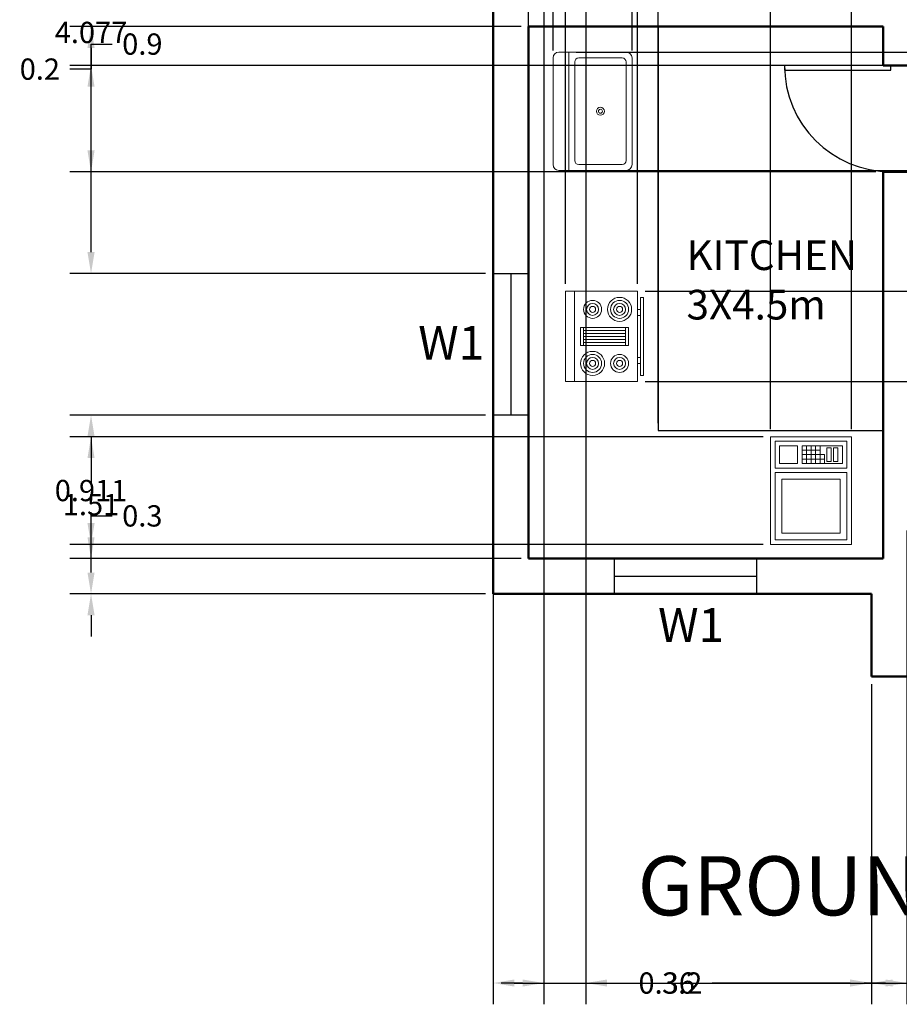
# Model space of a CAD drawing. Units: metres. Extents: x 2443.7 to 2482.9, y 2261.4 to 2287.
# Tile 1 of 8: x 2443.7 to 2451.1, y 2261.4 to 2269.7. Entities that reach past the tile are written whole.
import ezdxf

# ---------------------------------------------------------------- set-up
doc = ezdxf.new("R2010")
doc.units = ezdxf.units.M
for name, color, linetype, lineweight in [('A-ANNO-DIMS', 2, 'Continuous', 18), ('A-AREA-IDEN', 11, 'Continuous', 25), ('A-EQPM', 20, 'Continuous', 18), ('A-FLOR-CASE', 20, 'Continuous', 25), ('A-FLOR-FIXT', 20, 'Continuous', 18), ('A-MODL', 7, 'Continuous', 25), ('A-WALL', 7, 'Continuous', 50), ('door', 6, 'Continuous', 25), ('text', 11, 'Continuous', 25), ('window', 3, 'Continuous', 25)]:
    doc.layers.add(name, color=color, linetype=linetype, lineweight=lineweight)
doc.styles.get("Standard").update_dxf_attribs({"font": 'arial.ttf'})
doc.dimstyles.get("Standard").update_dxf_attribs({"dimtxt": 0.18, "dimasz": 0.18, "dimexe": 0.18, "dimexo": 0.0625, "dimgap": 0.09, "dimtad": 0, "dimtih": 1, "dimtoh": 1, "dimdec": 4, "dimzin": 0, "dimdsep": 46, "dimtxsty": 'Standard', "dimcen": 0.09, "dimadec": 0, "dimazin": 0, "dimtfac": 1, "dimtdec": 4, "dimtofl": 0, "dimtmove": 0, "dimatfit": 3, "dimfxl": 1, "dimtolj": 1, "dimtzin": 0, "dimarcsym": 0})

# ---------------------------------------------------------------- blocks, each defined once
blk = doc.blocks.new('*U2')
for p, q in [((0, 0), (0, -6)), ((-40, 0), (-40, -6))]:
    blk.add_line(p, q)
blk.add_lwpolyline([(0, 0), (0, 40), (-1.75, 40), (-1.75, 0)], close=True)
blk.add_arc((0, 0), 40, 90, 180)
blk = doc.blocks.new('Microwave')
for p, q in [((19, 7), (19, 11)), ((20, 11), (20, 7)), ((21, 7), (21, 11)), ((18, 10), (22, 10)), ((22, 9), (18, 9)), ((18, 8), (22, 8)), ((22, 7), (18, 7)), ((19, 6), (19, 7)), ((20, 7), (20, 6)), ((20, 6), (18, 6))]:
    blk.add_line(p, q)
for points in [[(0, 0), (0, 18), (24, 18), (24, 0)], [(1, 1), (1, 17), (16, 17), (16, 1)], [(2.5, 2.5), (2.5, 15.5), (14.5, 15.5), (14.5, 2.5)], [(17, 1), (17, 17), (23, 17), (23, 1)], [(18, 12), (18, 16), (22, 16), (22, 12)], [(18, 2), (18, 11), (22, 11), (22, 2)], [(18.5, 4.5), (18.5, 5.5), (21.5, 5.5), (21.5, 4.5)], [(18.5, 3), (18.5, 4), (21.5, 4), (21.5, 3)]]:
    blk.add_lwpolyline(points, close=True)
blk = doc.blocks.new('Range-Oven - 30 in top')
for p, q in [((0, -3), (30, -3)), ((12, -6), (18, -6)), ((13, -20), (13, -6)), ((14, -6), (14, -20)), ((15, -20), (15, -6)), ((16, -6), (16, -20)), ((17, -20), (17, -6)), ((18, -20), (12, -20)), ((6, -24), (6, -25)), ((8, -25), (8, -24)), ((22, -25), (22, -24)), ((24, -24), (24, -25))]:
    blk.add_line(p, q)
for points in [[(0, -24), (0, 0), (30, 0), (30, -24)], [(12, -21), (12, -5), (18, -5), (18, -21)], [(2, -26), (2, -25), (28, -25), (28, -26)]]:
    blk.add_lwpolyline(points, close=True)
for centre, radius in [((6, -9), 4), ((6, -9), 3), ((24, -9), 3), ((6, -9), 2), ((6, -9), 1), ((24, -9), 2), ((24, -9), 1), ((6, -18), 3), ((6, -18), 2), ((24, -18), 4), ((24, -18), 3), ((24, -18), 2), ((6, -18), 1), ((24, -18), 1)]:
    blk.add_circle(centre, radius)
blk = doc.blocks.new('Sink-single - 30 in top')
blk.add_line((-15, -3.999996), (15, -3.999996))
for points in [[(-13.5, 0), (13.5, 0)], [(-15, -18.499996), (-15, -1.5)], [(15, -1.5), (15, -18.499996)], [(-13.5, -17.499996), (-13.5, -6.499996)], [(-12.5, -5.499996), (12.5, -5.499996)], [(13.5, -6.499996), (13.5, -17.499996)], [(12.5, -18.499996), (-12.5, -18.499996)], [(13.5, -19.999996), (-13.5, -19.999996)]]:
    blk.add_lwpolyline(points)
for radius in [1, 0.5]:
    blk.add_circle((0, -11.999996), radius)
for centre, radius, start, end in [((-13.5, -1.5), 1.5, 90, 180), ((13.5, -1.5), 1.5, 0, 90), ((-12.5, -6.499996), 1, 90, 180), ((12.5, -6.499996), 1, 0, 90), ((-13.5, -18.499996), 1.5, 180, 270), ((-12.5, -17.499996), 1, 180, 270), ((12.5, -17.499996), 1, 270, 0), ((13.5, -18.499996), 1.5, 270, 0)]:
    blk.add_arc(centre, radius, start, end)
blk = doc.blocks.new('aditya')
at = {"layer": 'A-FLOR-CASE'}
for points in [[(1.3977, 0.3), (0.3, 0.3), (0.3, 4.8), (1.3977, 4.8), (1.3977, 1.3826)], [(1.3977, 1.3826), (3.3, 1.3826), (3.3, 0.3), (0.3, 0.3), (0.3, 1.3826)]]:
    blk.add_lwpolyline(points, dxfattribs=at)
at = {"layer": 'A-WALL'}
for p, q in [((0, 0), (0, 9.9)), ((0.3, 0.3), (0.3, 4.8)), ((0.3, 4.8), (3.3, 4.8)), ((3.3, 4.4718), (3.3, 4.8)), ((3.3, 0.3), (3.3, 3.5742)), ((0.3, 0.3), (3.3, 0.3)), ((0, 0), (3.2, 0)), ((3.2, -0.4), (3.2, 0)), ((3.2, -0.7), (3.2, 0)), ((3.5, -0.7), (3.2, -0.7))]:
    blk.add_line(p, q, dxfattribs=at)
for points in [[(3.3, 4.4718), (3.5, 4.4718)], [(3.5, 3.5718), (3.3, 3.5718), (3.3, 3.5742)]]:
    blk.add_lwpolyline(points, dxfattribs=at)
at = {"layer": 'window'}
for p, q in [((0.15, 2.7118), (0.15, 1.5118)), ((1.0287, 0.15), (2.2287, 0.15))]:
    blk.add_line(p, q, dxfattribs=at)
for points in [[(0, 2.7118), (0.3, 2.7118), (0.3, 1.5118), (0, 1.5118)], [(1.0287, 0), (1.0287, 0.3), (2.2287, 0.3), (2.2287, 0)]]:
    blk.add_lwpolyline(points, close=True, dxfattribs=at)
at = {"layer": 'A-EQPM', "rotation": 90}
for name, p, xscale, yscale, zscale in [('Range-Oven - 30 in top', (0.6135, 1.798), 0.0254, 0.0254, 0.0254), ('Microwave', (3.0315, 0.4191), 0.0379607650173663, 0.0379607650173663, 0.0379607650173663)]:
    blk.add_blockref(name, p, dxfattribs=dict(at, xscale=xscale, yscale=yscale, zscale=zscale))
at = {"layer": 'A-FLOR-FIXT', "xscale": 0.0333950198631644, "yscale": 0.0333950198631644, "zscale": 0.0333950198631644, "rotation": 90}
blk.add_blockref('Sink-single - 30 in top', (0.5076, 4.0837), dxfattribs=at)
at = {"layer": 'door', "xscale": 0.0224999999999983, "yscale": 0.0224999999999983, "zscale": 0.0224999999999983, "rotation": 90}
blk.add_blockref('*U2', (3.365, 4.4718), dxfattribs=at)
at = {"layer": 'A-AREA-IDEN', "insert": (1.6365, 2.991), "char_height": 0.250924, "attachment_point": 1}
blk.add_mtext_dynamic_manual_height_columns('{\\fArial|b1|i1|c0|p34;KITCHEN\\P3X4.5m}', width=10.569305, gutter_width=7.8414, heights=[0], dxfattribs=at)
at = {"layer": 'text'}
for p in [(-0.6327, 1.9824), (1.3964, -0.4055)]:
    blk.add_text('W1', height=0.28528, dxfattribs=at).set_placement(p)
at = {"layer": 'text', "insert": (1.2226, -2.2194), "char_height": 0.5, "attachment_point": 1}
blk.add_mtext_dynamic_manual_height_columns('{\\fArial|b1|i1|c0|p34;GROUND FLOOR PLAN}', width=17.015787, gutter_width=7.8414, heights=[0], dxfattribs=at)
blk = doc.blocks.new('*D22')
at = {"layer": 'A-ANNO-DIMS', "color": 0, "lineweight": -2, "transparency": 16777216}
for p, q in [((2457.8828, 2265.0972), (2457.8828, 2261.3876)), ((2447.6828, 2264.7972), (2447.6828, 2261.3876)), ((2447.8628, 2261.5676), (2452.4684, 2261.5676)), ((2457.7028, 2261.5676), (2453.0971, 2261.5676))]:
    blk.add_line(p, q, dxfattribs=at)
at = {"layer": 'A-ANNO-DIMS', "color": 0, "transparency": 16777216}
for points in [[(2447.8628, 2261.5976), (2447.8628, 2261.5376), (2447.6828, 2261.5676)], [(2457.7028, 2261.5976), (2457.7028, 2261.5376), (2457.8828, 2261.5676)]]:
    blk.add_solid(points, dxfattribs=at)
at = {"layer": 'Defpoints', "color": 0, "transparency": 16777216}
for p in [(2457.8828, 2265.1597), (2447.6828, 2264.8597), (2457.8828, 2261.5676)]:
    blk.add_point(p, dxfattribs=at)
at = {"layer": 'A-ANNO-DIMS', "color": 0, "transparency": 16777216, "insert": (2452.7828, 2261.5676), "char_height": 0.18, "attachment_point": 5}
blk.add_mtext('\\A1;10.2', dxfattribs=at)
blk = doc.blocks.new('*D24')
at = {"layer": 'A-ANNO-DIMS', "color": 0, "lineweight": -2, "transparency": 16777216}
for p, q in [((2447.6828, 2264.7972), (2447.6828, 2261.3876)), ((2450.8828, 2264.0972), (2450.8828, 2261.3876)), ((2447.8628, 2261.5676), (2449.0299, 2261.5676)), ((2450.7028, 2261.5676), (2449.5356, 2261.5676))]:
    blk.add_line(p, q, dxfattribs=at)
at = {"layer": 'A-ANNO-DIMS', "color": 0, "transparency": 16777216}
for points in [[(2447.8628, 2261.5976), (2447.8628, 2261.5376), (2447.6828, 2261.5676)], [(2450.7028, 2261.5976), (2450.7028, 2261.5376), (2450.8828, 2261.5676)]]:
    blk.add_solid(points, dxfattribs=at)
at = {"layer": 'Defpoints', "color": 0, "transparency": 16777216}
for p in [(2447.6828, 2264.8597), (2450.8828, 2264.1597), (2450.8828, 2261.5676)]:
    blk.add_point(p, dxfattribs=at)
at = {"layer": 'A-ANNO-DIMS', "color": 0, "transparency": 16777216, "insert": (2449.2828, 2261.5676), "char_height": 0.18, "attachment_point": 5}
blk.add_mtext('\\A1;3.2', dxfattribs=at)
blk = doc.blocks.new('*D25')
at = {"layer": 'A-ANNO-DIMS', "color": 0, "lineweight": -2, "transparency": 16777216}
for p, q in [((2450.8828, 2264.0972), (2450.8828, 2261.3876)), ((2453.5828, 2264.0972), (2453.5828, 2261.3876)), ((2451.0628, 2261.5676), (2451.9774, 2261.5676)), ((2453.4028, 2261.5676), (2452.4882, 2261.5676))]:
    blk.add_line(p, q, dxfattribs=at)
at = {"layer": 'A-ANNO-DIMS', "color": 0, "transparency": 16777216}
for points in [[(2451.0628, 2261.5976), (2451.0628, 2261.5376), (2450.8828, 2261.5676)], [(2453.4028, 2261.5976), (2453.4028, 2261.5376), (2453.5828, 2261.5676)]]:
    blk.add_solid(points, dxfattribs=at)
at = {"layer": 'Defpoints', "color": 0, "transparency": 16777216}
for p in [(2450.8828, 2264.1597), (2453.5828, 2264.1597), (2453.5828, 2261.5676)]:
    blk.add_point(p, dxfattribs=at)
at = {"layer": 'A-ANNO-DIMS', "color": 0, "transparency": 16777216, "insert": (2452.2328, 2261.5676), "char_height": 0.18, "attachment_point": 5}
blk.add_mtext('\\A1;2.7', dxfattribs=at)
blk = doc.blocks.new('*D31')
at = {"layer": 'A-ANNO-DIMS', "color": 0, "lineweight": -2, "transparency": 16777216}
for p, q in [((2447.6203, 2266.3715), (2444.1027, 2266.3715)), ((2444.2827, 2266.1915), (2444.2827, 2265.7975)), ((2444.2827, 2265.0397), (2444.2827, 2265.4337)), ((2447.6203, 2264.8597), (2444.1027, 2264.8597))]:
    blk.add_line(p, q, dxfattribs=at)
at = {"layer": 'A-ANNO-DIMS', "color": 0, "transparency": 16777216}
for points in [[(2444.2527, 2266.1915), (2444.3127, 2266.1915), (2444.2827, 2266.3715)], [(2444.2527, 2265.0397), (2444.3127, 2265.0397), (2444.2827, 2264.8597)]]:
    blk.add_solid(points, dxfattribs=at)
at = {"layer": 'Defpoints', "color": 0, "transparency": 16777216}
for p in [(2444.2827, 2266.3715), (2447.6828, 2266.3715), (2447.6828, 2264.8597)]:
    blk.add_point(p, dxfattribs=at)
at = {"layer": 'A-ANNO-DIMS', "color": 0, "transparency": 16777216, "insert": (2444.2827, 2265.6156), "char_height": 0.18, "attachment_point": 5}
blk.add_mtext('\\A1;1.51', dxfattribs=at)
blk = doc.blocks.new('*D32')
at = {"layer": 'A-ANNO-DIMS', "color": 0, "lineweight": -2, "transparency": 16777216}
for p, q in [((2447.6203, 2271.6487), (2444.1027, 2271.6487)), ((2444.2827, 2271.4687), (2444.2827, 2269.792)), ((2444.2827, 2267.7515), (2444.2827, 2269.4282)), ((2447.6203, 2267.5715), (2444.1027, 2267.5715))]:
    blk.add_line(p, q, dxfattribs=at)
at = {"layer": 'A-ANNO-DIMS', "color": 0, "transparency": 16777216}
for points in [[(2444.2527, 2271.4687), (2444.3127, 2271.4687), (2444.2827, 2271.6487)], [(2444.2527, 2267.7515), (2444.3127, 2267.7515), (2444.2827, 2267.5715)]]:
    blk.add_solid(points, dxfattribs=at)
at = {"layer": 'Defpoints', "color": 0, "transparency": 16777216}
for p in [(2444.2827, 2271.6487), (2447.6828, 2271.6487), (2447.6828, 2267.5715)]:
    blk.add_point(p, dxfattribs=at)
at = {"layer": 'A-ANNO-DIMS', "color": 0, "transparency": 16777216, "insert": (2444.2827, 2269.6101), "char_height": 0.18, "attachment_point": 5}
blk.add_mtext('\\A1;4.077', dxfattribs=at)
blk = doc.blocks.new('*D46')
at = {"layer": 'A-ANNO-DIMS', "color": 0, "lineweight": -2, "transparency": 16777216}
for p, q in [((2448.2963, 2267.4822), (2448.2963, 2287.0152)), ((2448.9059, 2267.4822), (2448.9059, 2287.0152)), ((2448.4763, 2286.8352), (2448.7259, 2286.8352)), ((2448.9059, 2286.8352), (2449.0859, 2286.8352))]:
    blk.add_line(p, q, dxfattribs=at)
at = {"layer": 'A-ANNO-DIMS', "color": 0, "transparency": 16777216}
for points in [[(2448.4763, 2286.8652), (2448.4763, 2286.8052), (2448.2963, 2286.8352)], [(2448.7259, 2286.8652), (2448.7259, 2286.8052), (2448.9059, 2286.8352)]]:
    blk.add_solid(points, dxfattribs=at)
at = {"layer": 'Defpoints', "color": 0, "transparency": 16777216}
for p in [(2448.9059, 2286.8352), (2448.2963, 2267.4197), (2448.9059, 2267.4197)]:
    blk.add_point(p, dxfattribs=at)
at = {"layer": 'A-ANNO-DIMS', "color": 0, "transparency": 16777216, "insert": (2449.3923, 2286.8352), "char_height": 0.18, "attachment_point": 5}
blk.add_mtext('\\A1;0.61', dxfattribs=at)
blk = doc.blocks.new('*D47')
at = {"layer": 'A-ANNO-DIMS', "color": 0, "lineweight": -2, "transparency": 16777216}
for p, q in [((2482.0628, 2267.4197), (2482.0628, 2267.5997)), ((2482.0628, 2267.5997), (2482.2428, 2267.5997)), ((2448.9684, 2267.4197), (2482.2428, 2267.4197)), ((2482.0628, 2266.8377), (2482.0628, 2267.2397)), ((2448.9684, 2266.6577), (2482.2428, 2266.6577))]:
    blk.add_line(p, q, dxfattribs=at)
at = {"layer": 'A-ANNO-DIMS', "color": 0, "transparency": 16777216}
for points in [[(2482.0328, 2267.2397), (2482.0928, 2267.2397), (2482.0628, 2267.4197)], [(2482.0328, 2266.8377), (2482.0928, 2266.8377), (2482.0628, 2266.6577)]]:
    blk.add_solid(points, dxfattribs=at)
at = {"layer": 'Defpoints', "color": 0, "transparency": 16777216}
for p in [(2448.9059, 2267.4197), (2482.0628, 2267.4197), (2448.9059, 2266.6577)]:
    blk.add_point(p, dxfattribs=at)
at = {"layer": 'A-ANNO-DIMS', "color": 0, "transparency": 16777216, "insert": (2482.6356, 2267.5997), "char_height": 0.18, "attachment_point": 5}
blk.add_mtext('\\A1;0.762', dxfattribs=at)
blk = doc.blocks.new('*D48')
at = {"layer": 'A-ANNO-DIMS', "color": 0, "lineweight": -2, "transparency": 16777216}
for p, q in [((2448.1904, 2269.4567), (2448.1904, 2287.0152)), ((2448.8583, 2269.4567), (2448.8583, 2287.0152)), ((2448.3704, 2286.8352), (2448.6783, 2286.8352)), ((2448.8583, 2286.8352), (2449.0383, 2286.8352))]:
    blk.add_line(p, q, dxfattribs=at)
at = {"layer": 'A-ANNO-DIMS', "color": 0, "transparency": 16777216}
for points in [[(2448.3704, 2286.8652), (2448.3704, 2286.8052), (2448.1904, 2286.8352)], [(2448.6783, 2286.8652), (2448.6783, 2286.8052), (2448.8583, 2286.8352)]]:
    blk.add_solid(points, dxfattribs=at)
at = {"layer": 'Defpoints', "color": 0, "transparency": 16777216}
for p in [(2448.8583, 2286.8352), (2448.1904, 2269.3942), (2448.8583, 2269.3942)]:
    blk.add_point(p, dxfattribs=at)
at = {"layer": 'A-ANNO-DIMS', "color": 0, "transparency": 16777216, "insert": (2449.4322, 2286.8352), "char_height": 0.18, "attachment_point": 5}
blk.add_mtext('\\A1;0.668', dxfattribs=at)
blk = doc.blocks.new('*D49')
at = {"layer": 'A-ANNO-DIMS', "color": 0, "lineweight": -2, "transparency": 16777216}
for p, q in [((2448.3865, 2269.4443), (2482.2428, 2269.4443)), ((2482.0628, 2269.2643), (2482.0628, 2269.1253)), ((2482.0628, 2268.6224), (2482.0628, 2268.7615)), ((2448.3865, 2268.4424), (2482.2428, 2268.4424))]:
    blk.add_line(p, q, dxfattribs=at)
at = {"layer": 'A-ANNO-DIMS', "color": 0, "transparency": 16777216}
for points in [[(2482.0328, 2269.2643), (2482.0928, 2269.2643), (2482.0628, 2269.4443)], [(2482.0328, 2268.6224), (2482.0928, 2268.6224), (2482.0628, 2268.4424)]]:
    blk.add_solid(points, dxfattribs=at)
at = {"layer": 'Defpoints', "color": 0, "transparency": 16777216}
for p in [(2448.324, 2269.4443), (2482.0628, 2269.4443), (2448.324, 2268.4424)]:
    blk.add_point(p, dxfattribs=at)
at = {"layer": 'A-ANNO-DIMS', "color": 0, "transparency": 16777216, "insert": (2482.0628, 2268.9434), "char_height": 0.18, "attachment_point": 5}
blk.add_mtext('\\A1;1.00', dxfattribs=at)
blk = doc.blocks.new('*D50')
at = {"layer": 'A-ANNO-DIMS', "color": 0, "lineweight": -2, "transparency": 16777216}
for p, q in [((2450.031, 2266.2523), (2450.031, 2287.0152)), ((2450.7143, 2266.2523), (2450.7143, 2287.0152)), ((2449.851, 2286.8352), (2449.671, 2286.8352)), ((2450.8943, 2286.8352), (2451.0743, 2286.8352))]:
    blk.add_line(p, q, dxfattribs=at)
at = {"layer": 'A-ANNO-DIMS', "color": 0, "transparency": 16777216}
for points in [[(2449.851, 2286.8652), (2449.851, 2286.8052), (2450.031, 2286.8352)], [(2450.8943, 2286.8652), (2450.8943, 2286.8052), (2450.7143, 2286.8352)]]:
    blk.add_solid(points, dxfattribs=at)
at = {"layer": 'Defpoints', "color": 0, "transparency": 16777216}
for p in [(2450.7143, 2286.8352), (2450.031, 2266.1898), (2450.7143, 2266.1898)]:
    blk.add_point(p, dxfattribs=at)
at = {"layer": 'A-ANNO-DIMS', "color": 0, "transparency": 16777216, "insert": (2450.3726, 2286.8352), "char_height": 0.18, "attachment_point": 5}
blk.add_mtext('\\A1;0.68', dxfattribs=at)
blk = doc.blocks.new('*D51')
at = {"layer": 'A-ANNO-DIMS', "color": 0, "lineweight": -2, "transparency": 16777216}
for p, q in [((2449.9685, 2266.1898), (2444.1027, 2266.1898)), ((2444.2827, 2266.0098), (2444.2827, 2265.9162)), ((2444.2827, 2265.4588), (2444.2827, 2265.5524)), ((2449.9685, 2265.2788), (2444.1027, 2265.2788))]:
    blk.add_line(p, q, dxfattribs=at)
at = {"layer": 'A-ANNO-DIMS', "color": 0, "transparency": 16777216}
for points in [[(2444.2527, 2266.0098), (2444.3127, 2266.0098), (2444.2827, 2266.1898)], [(2444.2527, 2265.4588), (2444.3127, 2265.4588), (2444.2827, 2265.2788)]]:
    blk.add_solid(points, dxfattribs=at)
at = {"layer": 'Defpoints', "color": 0, "transparency": 16777216}
for p in [(2444.2827, 2266.1898), (2450.031, 2266.1898), (2450.031, 2265.2788)]:
    blk.add_point(p, dxfattribs=at)
at = {"layer": 'A-ANNO-DIMS', "color": 0, "transparency": 16777216, "insert": (2444.2827, 2265.7343), "char_height": 0.18, "attachment_point": 5}
blk.add_mtext('\\A1;0.911', dxfattribs=at)
blk = doc.blocks.new('*D52')
at = {"layer": 'A-ANNO-DIMS', "color": 0, "lineweight": -2, "transparency": 16777216}
for p, q in [((2451.182762, 2265.397173), (2451.182762, 2261.387605)), ((2452.042262, 2265.397173), (2452.042262, 2261.387605)), ((2451.002762, 2261.567605), (2450.822762, 2261.567605)), ((2452.222262, 2261.567605), (2452.402262, 2261.567605))]:
    blk.add_line(p, q, dxfattribs=at)
at = {"layer": 'A-ANNO-DIMS', "color": 0, "transparency": 16777216}
for points in [[(2451.002762, 2261.597605), (2451.002762, 2261.537605), (2451.182762, 2261.567605)], [(2452.222262, 2261.597605), (2452.222262, 2261.537605), (2452.042262, 2261.567605)]]:
    blk.add_solid(points, dxfattribs=at)
at = {"layer": 'Defpoints', "color": 0, "transparency": 16777216}
for p in [(2451.182762, 2265.459673), (2452.042262, 2265.459673), (2452.042262, 2261.567605)]:
    blk.add_point(p, dxfattribs=at)
at = {"layer": 'A-ANNO-DIMS', "color": 0, "transparency": 16777216, "insert": (2451.612512, 2261.567605), "char_height": 0.18, "attachment_point": 5}
blk.add_mtext('\\A1;0.86', dxfattribs=at)
blk = doc.blocks.new('*D53')
at = {"layer": 'A-ANNO-DIMS', "color": 0, "lineweight": -2, "transparency": 16777216}
for p, q in [((2444.2827, 2269.3315), (2444.2827, 2269.5115)), ((2444.2827, 2269.5115), (2444.4627, 2269.5115)), ((2450.9203, 2269.3315), (2444.1027, 2269.3315)), ((2444.2827, 2268.6115), (2444.2827, 2269.1515)), ((2450.9203, 2268.4315), (2444.1027, 2268.4315))]:
    blk.add_line(p, q, dxfattribs=at)
at = {"layer": 'A-ANNO-DIMS', "color": 0, "transparency": 16777216}
for points in [[(2444.2527, 2269.1515), (2444.3127, 2269.1515), (2444.2827, 2269.3315)], [(2444.2527, 2268.6115), (2444.3127, 2268.6115), (2444.2827, 2268.4315)]]:
    blk.add_solid(points, dxfattribs=at)
at = {"layer": 'Defpoints', "color": 0, "transparency": 16777216}
for p in [(2444.2827, 2269.3315), (2450.9828, 2269.3315), (2450.9828, 2268.4315)]:
    blk.add_point(p, dxfattribs=at)
at = {"layer": 'A-ANNO-DIMS', "color": 0, "transparency": 16777216, "insert": (2444.7168, 2269.5115), "char_height": 0.18, "attachment_point": 5}
blk.add_mtext('\\A1;0.9', dxfattribs=at)
blk = doc.blocks.new('*D59')
at = {"layer": 'A-ANNO-DIMS', "color": 0, "lineweight": -2, "transparency": 16777216}
for p, q in [((2448.1123, 2274.0125), (2448.1123, 2261.3876)), ((2448.4679, 2274.0125), (2448.4679, 2261.3876)), ((2447.9323, 2261.5676), (2447.7523, 2261.5676)), ((2448.6479, 2261.5676), (2448.8279, 2261.5676))]:
    blk.add_line(p, q, dxfattribs=at)
at = {"layer": 'A-ANNO-DIMS', "color": 0, "transparency": 16777216}
for points in [[(2447.9323, 2261.5976), (2447.9323, 2261.5376), (2448.1123, 2261.5676)], [(2448.6479, 2261.5976), (2448.6479, 2261.5376), (2448.4679, 2261.5676)]]:
    blk.add_solid(points, dxfattribs=at)
at = {"layer": 'Defpoints', "color": 0, "transparency": 16777216}
for p in [(2448.1123, 2274.075), (2448.4679, 2274.075), (2448.4679, 2261.5676)]:
    blk.add_point(p, dxfattribs=at)
at = {"layer": 'A-ANNO-DIMS', "color": 0, "transparency": 16777216, "insert": (2449.1516, 2261.5676), "char_height": 0.18, "attachment_point": 5}
blk.add_mtext('\\A1;0.36', dxfattribs=at)
blk = doc.blocks.new('*D60')
at = {"layer": 'A-ANNO-DIMS', "color": 0, "lineweight": -2, "transparency": 16777216}
for p, q in [((2444.2827, 2265.3397), (2444.2827, 2265.5197)), ((2444.2827, 2265.5197), (2444.4627, 2265.5197)), ((2447.9203, 2265.1597), (2444.1027, 2265.1597)), ((2447.6203, 2264.8597), (2444.1027, 2264.8597)), ((2444.2827, 2264.6797), (2444.2827, 2264.4997))]:
    blk.add_line(p, q, dxfattribs=at)
at = {"layer": 'A-ANNO-DIMS', "color": 0, "transparency": 16777216}
for points in [[(2444.2527, 2265.3397), (2444.3127, 2265.3397), (2444.2827, 2265.1597)], [(2444.2527, 2264.6797), (2444.3127, 2264.6797), (2444.2827, 2264.8597)]]:
    blk.add_solid(points, dxfattribs=at)
at = {"layer": 'Defpoints', "color": 0, "transparency": 16777216}
for p in [(2444.2827, 2265.1597), (2447.9828, 2265.1597), (2447.6828, 2264.8597)]:
    blk.add_point(p, dxfattribs=at)
at = {"layer": 'A-ANNO-DIMS', "color": 0, "transparency": 16777216, "insert": (2444.7166, 2265.5197), "char_height": 0.18, "attachment_point": 5}
blk.add_mtext('\\A1;0.3', dxfattribs=at)
blk = doc.blocks.new('*D61')
at = {"layer": 'A-ANNO-DIMS', "color": 0, "lineweight": -2, "transparency": 16777216}
for p, q in [((2444.2827, 2270.0397), (2444.2827, 2270.2197)), ((2447.9203, 2269.8597), (2444.1027, 2269.8597)), ((2447.9203, 2269.6597), (2444.1027, 2269.6597)), ((2444.2827, 2269.4797), (2444.2827, 2269.2997)), ((2444.2827, 2269.2997), (2444.1027, 2269.2997))]:
    blk.add_line(p, q, dxfattribs=at)
at = {"layer": 'A-ANNO-DIMS', "color": 0, "transparency": 16777216}
for points in [[(2444.2527, 2270.0397), (2444.3127, 2270.0397), (2444.2827, 2269.8597)], [(2444.2527, 2269.4797), (2444.3127, 2269.4797), (2444.2827, 2269.6597)]]:
    blk.add_solid(points, dxfattribs=at)
at = {"layer": 'Defpoints', "color": 0, "transparency": 16777216}
for p in [(2447.9828, 2269.8597), (2444.2827, 2269.6597), (2447.9828, 2269.6597)]:
    blk.add_point(p, dxfattribs=at)
at = {"layer": 'A-ANNO-DIMS', "color": 0, "transparency": 16777216, "insert": (2443.8498, 2269.2997), "char_height": 0.18, "attachment_point": 5}
blk.add_mtext('\\A1;0.2', dxfattribs=at)
blk = doc.blocks.new('*D62')
at = {"layer": 'A-ANNO-DIMS', "color": 0, "lineweight": -2, "transparency": 16777216}
for p, q in [((2447.982762, 2265.222173), (2447.982762, 2287.015188)), ((2449.080462, 2266.304727), (2449.080462, 2287.015188)), ((2447.802762, 2286.835188), (2447.622762, 2286.835188)), ((2449.260462, 2286.835188), (2449.440462, 2286.835188))]:
    blk.add_line(p, q, dxfattribs=at)
at = {"layer": 'A-ANNO-DIMS', "color": 0, "transparency": 16777216}
for points in [[(2447.802762, 2286.865188), (2447.802762, 2286.805188), (2447.982762, 2286.835188)], [(2449.260462, 2286.865188), (2449.260462, 2286.805188), (2449.080462, 2286.835188)]]:
    blk.add_solid(points, dxfattribs=at)
at = {"layer": 'Defpoints', "color": 0, "transparency": 16777216}
for p in [(2449.080462, 2286.835188), (2449.080462, 2266.242227), (2447.982762, 2265.159673)]:
    blk.add_point(p, dxfattribs=at)
at = {"layer": 'A-ANNO-DIMS', "color": 0, "transparency": 16777216, "insert": (2448.531612, 2286.835188), "char_height": 0.18, "attachment_point": 5}
blk.add_mtext('\\A1;1.10', dxfattribs=at)
blk = doc.blocks.new('*D63')
at = {"layer": 'A-ANNO-DIMS', "color": 0, "lineweight": -2, "transparency": 16777216}
for p, q in [((2447.6828, 2278.9987), (2447.6828, 2261.3876)), ((2457.8828, 2278.9987), (2457.8828, 2261.3876)), ((2447.8628, 2261.5676), (2452.4684, 2261.5676)), ((2457.7028, 2261.5676), (2453.0971, 2261.5676))]:
    blk.add_line(p, q, dxfattribs=at)
at = {"layer": 'A-ANNO-DIMS', "color": 0, "transparency": 16777216}
for points in [[(2447.8628, 2261.5976), (2447.8628, 2261.5376), (2447.6828, 2261.5676)], [(2457.7028, 2261.5976), (2457.7028, 2261.5376), (2457.8828, 2261.5676)]]:
    blk.add_solid(points, dxfattribs=at)
at = {"layer": 'Defpoints', "color": 0, "transparency": 16777216}
for p in [(2447.6828, 2279.0612), (2457.8828, 2279.0612), (2457.8828, 2261.5676)]:
    blk.add_point(p, dxfattribs=at)
at = {"layer": 'A-ANNO-DIMS', "color": 0, "transparency": 16777216, "insert": (2452.7828, 2261.5676), "char_height": 0.18, "attachment_point": 5}
blk.add_mtext('\\A1;10.2', dxfattribs=at)

msp = doc.modelspace()

# ---------------------------------------------------------------- block references
at = {"layer": 'A-MODL'}
msp.add_blockref('aditya', (2447.682762, 2264.859673), dxfattribs=at)

# ---------------------------------------------------------------- dimensions: what is measured, and where the dimension line sits
at = {"layer": 'A-ANNO-DIMS'}
for base, p1, p2, override, picture, middle in [((2449.080462, 2286.835188), (2447.982762, 2265.159673), (2449.080462, 2266.242227), {"dimdec": 2, "dimlfac": 1, "dimrnd": 0, "dimzin": 0, "dimdsep": 46, "dimlunit": 2}, '*D62', (2448.531612, 2286.835188)), ((2448.858297, 2286.835188), (2448.190396, 2269.394205), (2448.858297, 2269.394205), {"dimdec": 3, "dimlfac": 1, "dimrnd": 0, "dimzin": 0, "dimdsep": 46, "dimlunit": 2}, '*D48', (2449.432185, 2286.835188)), ((2448.905882, 2286.835188), (2448.296282, 2267.419676), (2448.905882, 2267.419676), {"dimdec": 2, "dimlfac": 1, "dimrnd": 0, "dimzin": 0, "dimdsep": 46, "dimlunit": 2}, '*D46', (2449.392287, 2286.835188)), ((2450.714284, 2286.835188), (2450.030991, 2266.189812), (2450.714284, 2266.189812), {"dimdec": 2, "dimlfac": 1, "dimrnd": 0, "dimzin": 0, "dimdsep": 46, "dimlunit": 2}, '*D50', (2450.372638, 2286.835188)), ((2457.882762, 2261.567605), (2447.682762, 2279.061188), (2457.882762, 2279.061188), {"dimdec": 1, "dimlfac": 1, "dimrnd": 0, "dimzin": 0, "dimdsep": 46, "dimlunit": 2}, '*D63', (2452.782762, 2261.567605)), ((2448.467902, 2261.567605), (2448.112302, 2274.07505), (2448.467902, 2274.07505), {"dimdec": 2, "dimlfac": 1, "dimrnd": 0, "dimzin": 0, "dimdsep": 46, "dimlunit": 2}, '*D59', (2449.15162, 2261.567605)), ((2452.042262, 2261.567605), (2451.182762, 2265.459673), (2452.042262, 2265.459673), {"dimdec": 2, "dimlfac": 1, "dimrnd": 0, "dimzin": 0, "dimdsep": 46, "dimlunit": 2}, '*D52', (2451.612512, 2261.567605)), ((2457.882762, 2261.567605), (2447.682762, 2264.859673), (2457.882762, 2265.159673), {"dimdec": 1, "dimlfac": 1, "dimrnd": 0, "dimzin": 0, "dimdsep": 46, "dimlunit": 2}, '*D22', (2452.782762, 2261.567605)), ((2450.882762, 2261.567605), (2447.682762, 2264.859673), (2450.882762, 2264.159673), {"dimdec": 1, "dimlfac": 1, "dimrnd": 0, "dimzin": 0, "dimdsep": 46, "dimlunit": 2}, '*D24', (2449.282762, 2261.567605)), ((2453.582762, 2261.567605), (2450.882762, 2264.159673), (2453.582762, 2264.159673), {"dimdec": 1, "dimlfac": 1, "dimrnd": 0, "dimzin": 0, "dimdsep": 46, "dimlunit": 2}, '*D25', (2452.232762, 2261.567605))]:
    dim = msp.add_linear_dim(base=base, p1=p1, p2=p2, dimstyle='Standard', override=override, dxfattribs=at)
    dim.commit()
    dim.dimension.update_dxf_attribs({"geometry": picture, "text_midpoint": middle})
for base, p1, p2, override, picture, middle in [((2444.282724, 2271.648723), (2447.682762, 2267.571466), (2447.682762, 2271.648723), {"dimdec": 3, "dimlfac": 1, "dimrnd": 0, "dimzin": 0, "dimdsep": 46, "dimlunit": 2}, '*D32', (2444.282724, 2269.610094)), ((2444.282724, 2269.659673), (2447.982762, 2269.859673), (2447.982762, 2269.659673), {"dimdec": 1, "dimlfac": 1, "dimrnd": 0, "dimzin": 0, "dimdsep": 46, "dimlunit": 2}, '*D61', (2443.849791, 2269.299673)), ((2444.282724, 2269.331522), (2450.982762, 2268.431522), (2450.982762, 2269.331522), {"dimdec": 1, "dimlfac": 1, "dimrnd": 0, "dimzin": 0, "dimdsep": 46, "dimlunit": 2}, '*D53', (2444.716762, 2269.511522)), ((2482.062768, 2269.444297), (2448.323976, 2268.442446), (2448.323976, 2269.444297), {"dimdec": 2, "dimlfac": 1, "dimrnd": 0, "dimzin": 0, "dimdsep": 46, "dimlunit": 2}, '*D49', (2482.062768, 2268.943372)), ((2482.062768, 2267.419676), (2448.905882, 2266.657676), (2448.905882, 2267.419676), {"dimdec": 3, "dimlfac": 1, "dimrnd": 0, "dimzin": 0, "dimdsep": 46, "dimlunit": 2}, '*D47', (2482.635551, 2267.599676)), ((2444.282724, 2266.371466), (2447.682762, 2264.859673), (2447.682762, 2266.371466), {"dimdec": 2, "dimlfac": 1, "dimrnd": 0, "dimzin": 0, "dimdsep": 46, "dimlunit": 2}, '*D31', (2444.282724, 2265.61557)), ((2444.282724, 2266.189812), (2450.030991, 2265.278754), (2450.030991, 2266.189812), {"dimdec": 3, "dimlfac": 1, "dimrnd": 0, "dimzin": 0, "dimdsep": 46, "dimlunit": 2}, '*D51', (2444.282724, 2265.734283)), ((2444.282724, 2265.159673), (2447.682762, 2264.859673), (2447.982762, 2265.159673), {"dimdec": 1, "dimlfac": 1, "dimrnd": 0, "dimzin": 0, "dimdsep": 46, "dimlunit": 2}, '*D60', (2444.716578, 2265.519673))]:
    dim = msp.add_linear_dim(base=base, p1=p1, p2=p2, angle=90, dimstyle='Standard', override=override, dxfattribs=at)
    dim.commit()
    dim.dimension.update_dxf_attribs({"geometry": picture, "text_midpoint": middle})

doc.saveas('drawing.dxf')
